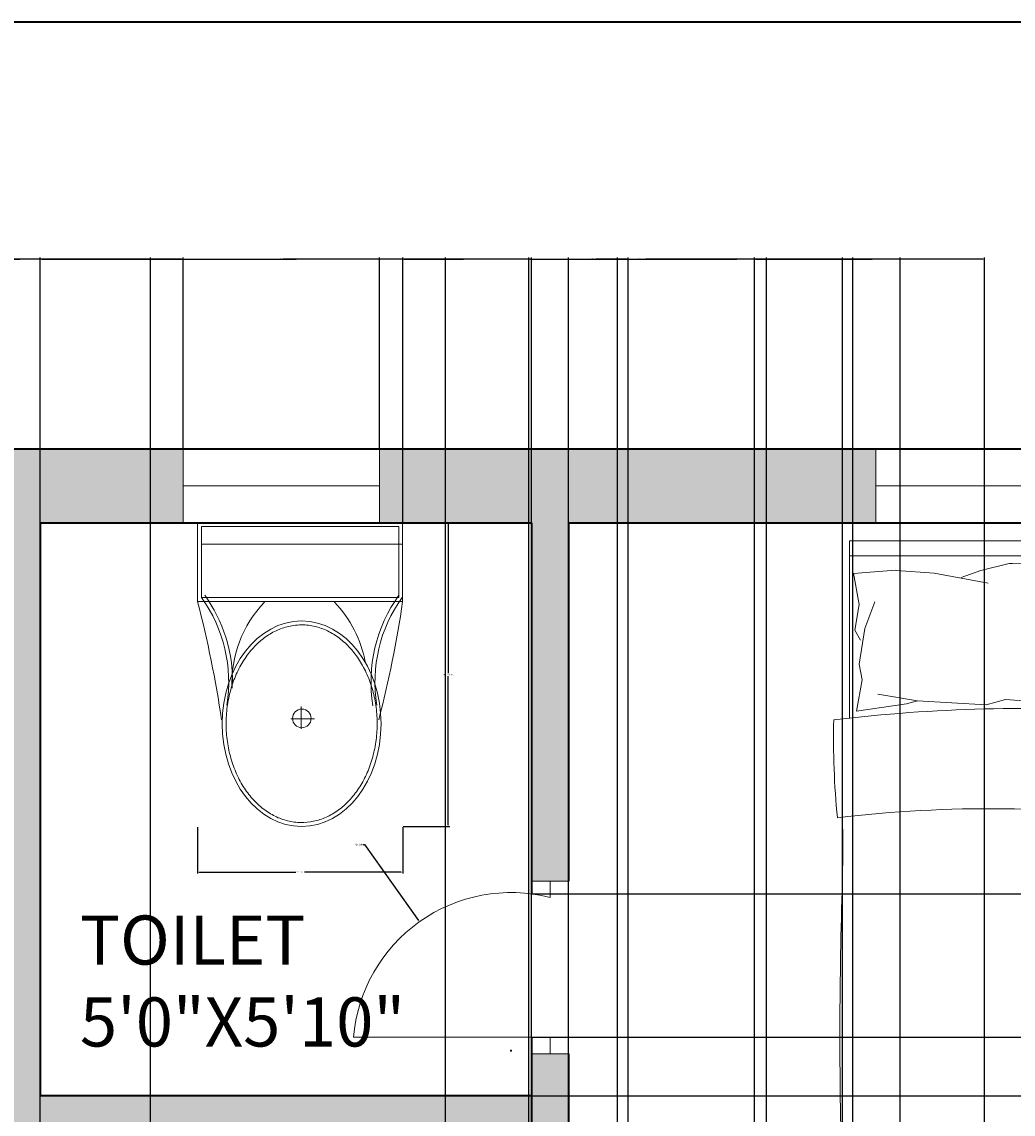
# Model space of a CAD drawing. Units: inches. Extents: x 2606 to 3027, y 1906 to 2463.
# Tile 9 of 10: x 2785 to 2906, y 2329 to 2463. Entities that reach past the tile are written whole.
import ezdxf

# ---------------------------------------------------------------- set-up
doc = ezdxf.new("R2010")
doc.units = ezdxf.units.IN
for name, color, linetype, lineweight in [('A-ANNO-DIMS', 2, 'Continuous', 18), ('A-ANNO-TTLB', 7, 'Continuous', 35), ('A-AREA-IDEN', 7, 'Continuous', 18), ('A-DOOR', 3, 'Continuous', 18), ('A-FLOR-FIXT', 9, 'Continuous', 18), ('A-FURN', 8, 'Continuous', 13), ('A-GLAZ', 4, 'Continuous', 18), ('A-WALL', 7, 'Continuous', 35)]:
    doc.layers.add(name, color=color, linetype=linetype, lineweight=lineweight)
doc.layers.add('A-WALL-PATT', color=251, linetype='Continuous', lineweight=13, true_color=0x636466)
doc.styles.get("Standard").update_dxf_attribs({"font": 'arial.ttf'})
doc.dimstyles.get("Standard").update_dxf_attribs({"dimtxt": 0.18, "dimasz": 0.18, "dimexe": 0.18, "dimexo": 0.0625, "dimgap": 0.09, "dimtad": 0, "dimtih": 1, "dimtoh": 1, "dimdec": 4, "dimzin": 0, "dimdsep": 46, "dimtxsty": 'Standard', "dimcen": 0.09, "dimadec": 0, "dimazin": 0, "dimtfac": 1, "dimtdec": 4, "dimtofl": 0, "dimtmove": 0, "dimatfit": 3, "dimfxl": 1, "dimtolj": 1, "dimtzin": 0, "dimarcsym": 0})

# ---------------------------------------------------------------- blocks, each defined once
blk = doc.blocks.new('A$C31115884')
for p, q in [((257.5, 466.4), (257.5, 523.2)), ((283.1, 497.7), (223.4, 497.7)), ((0, 200), (0, 0)), ((520, 200), (0, 200)), ((520, 0), (520, 200)), ((10, 190), (10, 10)), ((510, 190), (10, 190)), ((510, 10), (510, 190)), ((510, 54.5), (0, 54.5)), ((10, 10), (510, 10)), ((0, 0), (520, 0))]:
    blk.add_line(p, q)
blk.add_circle((255.6, 496.4), 23.6)
for centre, radius, start, end in [((2777.7, -204.6), 2807, 165.4549, 171.7133), ((3237, 905), 2807, 188.2867, 194.5451), ((-294.5, 403.3), 364.7, 324.2091, 9.3499), ((-294.5, 403.3), 374.7, 324.2091, 9.3499), ((805.8, 403.3), 364.7, 170.6501, 215.7909), ((139.5, 406.2), 293.5, 315.8436, 2.6563), ((805.8, 403.3), 374.7, 179.2036, 215.7909), ((383.6, 406.2), 293.5, 190.2774, 224.1564)]:
    blk.add_arc(centre, radius, start, end)
blk.add_ellipse((256.2, 509.9), major_axis=(0, -260.7), ratio=0.772727)
blk.add_open_spline([(256.2, 259.2), (263.1, 259.2), (270, 259.7), (287.8, 262.3), (298.7, 265.1), (319.9, 273.1), (330.2, 278.4), (350.1, 291.1), (359.7, 298.7), (377.7, 315.9), (386.2, 325.5), (401.7, 346.6), (408.8, 358.1), (421.3, 382.5), (426.8, 395.5), (435.9, 422.4), (439.5, 436.4), (444.8, 465.1), (446.5, 479.7), (447.9, 509.2), (447.6, 524), (445, 553.3), (442.7, 567.8), (436.3, 596), (432.1, 609.7), (421.9, 636), (416, 648.6), (402.5, 672.1), (395, 683), (378.6, 703), (369.8, 712.1), (351.1, 728), (341.3, 734.8), (320.9, 746.2), (310.4, 750.7), (288.9, 757.3), (278, 759.4), (256, 761), (245, 760.6), (223.1, 757.2), (212.3, 754.3), (191.1, 746.1), (180.8, 740.7), (160.9, 727.8), (151.4, 720.1), (133.5, 702.7), (125.1, 693), (109.6, 671.7), (102.6, 660.2), (90.2, 635.7), (84.9, 622.7), (76, 595.6), (72.4, 581.6), (67.2, 552.9), (65.6, 538.2), (64.4, 508.8), (64.8, 494), (67.5, 464.7), (69.9, 450.2), (76.6, 422), (80.8, 408.3), (91.1, 382.2), (97.2, 369.7), (110.8, 346.3), (118.4, 335.4), (134.8, 315.6), (143.7, 306.7), (162.4, 290.9), (172.3, 284.2), (192.8, 273), (203.3, 268.6), (224.8, 262.2), (235.8, 260.2), (249.9, 259.3), (253, 259.2), (256.2, 259.2)], degree=3, knots=[0, 0, 0, 0, 0.110105, 0.110105, 0.285049, 0.285049, 0.459994, 0.459994, 0.634938, 0.634938, 0.809882, 0.809882, 0.984827, 0.984827, 1.159771, 1.159771, 1.334715, 1.334715, 1.50966, 1.50966, 1.684604, 1.684604, 1.859549, 1.859549, 2.034493, 2.034493, 2.209437, 2.209437, 2.384382, 2.384382, 2.559326, 2.559326, 2.73427, 2.73427, 2.909215, 2.909215, 3.084159, 3.084159, 3.259103, 3.259103, 3.434048, 3.434048, 3.608992, 3.608992, 3.783936, 3.783936, 3.958881, 3.958881, 4.133825, 4.133825, 4.30877, 4.30877, 4.483714, 4.483714, 4.658658, 4.658658, 4.833603, 4.833603, 5.008547, 5.008547, 5.183491, 5.183491, 5.358436, 5.358436, 5.53338, 5.53338, 5.708324, 5.708324, 5.883269, 5.883269, 6.058213, 6.058213, 6.233158, 6.233158, 6.283185, 6.283185, 6.283185, 6.283185])
blk = doc.blocks.new('BED-DOUBLE')
for p, q in [((4.17, 75.16), (4.17, 96.87)), ((4.17, 96.87), (61.46, 96.87)), ((61.46, 96.87), (61.46, 64.97)), ((4.17, 95.03), (61.46, 95.03)), ((20.24, 93.24), (23.7, 94.11)), ((23.7, 94.11), (24.09, 94.11)), ((24.09, 94.11), (29.42, 93.94)), ((29.42, 93.94), (31.15, 94.63)), ((31.15, 94.63), (31.84, 88.22)), ((33.54, 93.89), (33.25, 87.44)), ((35.31, 93.3), (33.54, 93.89)), ((40.62, 93.81), (35.31, 93.3)), ((41.01, 93.83), (40.62, 93.81)), ((44.52, 93.18), (41.01, 93.83)), ((54.8, 93.82), (50.25, 93.19)), ((60.08, 93.81), (53.6, 93.92)), ((53.6, 93.92), (54.8, 93.82)), ((60.08, 93.81), (59.62, 89.96)), ((4.67, 92.87), (9.81, 93.27)), ((4.67, 92.9), (5.36, 89.08)), ((9.81, 93.27), (9.93, 93.24)), ((9.93, 93.24), (14.52, 92.9)), ((14.52, 92.9), (21.1, 91.68)), ((17.81, 92.38), (20.24, 93.24)), ((50.25, 93.19), (43.75, 91.57)), ((47, 92.47), (44.52, 93.18)), ((6.06, 86.14), (7.27, 89.43)), ((59.12, 86.97), (57.7, 90.18)), ((59.62, 89.96), (60.34, 86.88)), ((5.36, 89.08), (4.84, 85.96)), ((31.84, 88.22), (32.54, 84.4)), ((33.25, 87.44), (32.79, 83.59)), ((60.08, 82.69), (59.12, 86.97)), ((60.34, 86.88), (59.72, 85.62)), ((4.84, 85.96), (5.54, 84.75)), ((5.36, 81.8), (6.06, 86.14)), ((32.54, 84.4), (32.54, 82.84)), ((32.54, 82.84), (31.84, 80.59)), ((32.79, 83.59), (32.89, 82.03)), ((5.71, 79.9), (5.36, 81.8)), ((32.89, 82.03), (33.72, 79.83)), ((59.85, 80.77), (60.08, 82.69)), ((31.84, 80.59), (31.84, 77.38)), ((60.78, 77), (59.85, 80.77)), ((5.02, 76.08), (5.71, 79.9)), ((33.72, 79.83), (33.92, 76.62)), ((7.65, 78.14), (12.48, 77.34)), ((20.89, 76.82), (23.24, 77.49)), ((23.24, 77.49), (29.39, 77)), ((28.9, 77.38), (25.13, 78.68)), ((36.87, 76.8), (40.55, 78.34)), ((39.04, 78.14), (43.87, 77.34)), ((52.28, 76.82), (54.63, 77.49)), ((54.63, 77.49), (60.78, 77)), ((11.13, 76.95), (5.02, 76.08)), ((12.48, 77.34), (11.13, 76.95)), ((12.48, 77.34), (20.89, 76.82)), ((31.84, 77.38), (28.9, 77.38)), ((33.92, 76.62), (36.87, 76.8)), ((43.87, 77.34), (52.28, 76.82)), ((36.28, 76.03), (41.3, 68.25)), ((48.73, 72.52), (38.73, 76.03)), ((55.41, 70.1), (48.73, 72.52)), ((58.94, 67.51), (55.41, 70.1)), ((41.3, 68.25), (43.34, 62.87)), ((63.38, 63.61), (58.94, 67.51)), ((43.34, 62.87), (43.71, 60.45)), ((49.1, 62.31), (53.18, 62.87)), ((53.18, 62.87), (57.82, 63.24)), ((57.82, 63.24), (61.54, 62.87)), ((61.54, 62.87), (63.38, 63.61)), ((63.48, 61.52), (63.38, 63.61, 4.64)), ((46.68, 61.2), (49.1, 62.31)), ((43.71, 60.45), (46.68, 61.2)), ((18.06, 1.87), (47.57, 1.87))]:
    blk.add_line(p, q)
for centre, radius, start, end in [((25.61, -121.38), 197.77, 86.0865, 96.7821), ((102.1, 72.78), 99.87, 178.7218, 185.604), ((21.29, -90.53), 154.68, 81.7845, 96.9006), ((-200.58, 59.5), 203.94, 358.4762, 1.0082), ((37.35, 95.1), 35.55, 280.6617, 289.8806), ((52.44, 54.83), 7.46, 78.6608, 113.7384), ((61.53, 104.85), 43.38, 259.8763, 272.5657), ((218.51, 53.34), 155.25, 176.9791, 183.8365), ((43.92, 60.38), 0.221, 160.2464, 271.1377), ((581.23, 36.19), 578.22, 178.22771, 181.71854), ((-5405.34, 15.56), 5469.02, 0.00217, 0.28689), ((-32.25, 19.53), 35.53, 346.0648, 358.9113), ((91.3, 14.55), 27.65, 177.4714, 206.4681), ((-25.97, 12.62), 28.25, 337.9751, 356.652), ((-20.65, 125.3), 127.63, 283.3832, 287.7053), ((1.3, 1.3), 1.31, 146.1736, 293.4781), ((25.69, -143.9), 145.97, 92.9958, 99.4091), ((49.34, -157.62), 159.5, 84.4998, 90.6351), ((65.23, 2.32), 1.32, 242.6588, 356.02)]:
    blk.add_arc(centre, radius, start, end)
blk = doc.blocks.new('WIN-60IN')
for p, q in [((0, 9), (0, 0)), ((60, 4.5), (60, 9)), ((60, 9), (60, 0)), ((0, 0), (0, 4.5)), ((0, 4.5), (60, 4.5))]:
    blk.add_line(p, q)
blk = doc.blocks.new('*D15')
at = {"layer": 'A-ANNO-DIMS', "color": 0, "lineweight": -2, "transparency": 16777216}
for p, q in [((2831.88, 2401.61), (2837.56, 2401.61)), ((2837.38, 2401.43), (2837.38, 2383.24)), ((2837.38, 2364.68), (2837.38, 2382.87)), ((2831.88, 2364.5), (2837.56, 2364.5))]:
    blk.add_line(p, q, dxfattribs=at)
at = {"layer": 'A-ANNO-DIMS', "color": 0, "transparency": 16777216}
for points in [[(2837.35, 2401.43), (2837.41, 2401.43), (2837.38, 2401.61)], [(2837.35, 2364.68), (2837.41, 2364.68), (2837.38, 2364.5)]]:
    blk.add_solid(points, dxfattribs=at)
at = {"layer": 'Defpoints', "color": 0, "transparency": 16777216}
for p in [(2831.82, 2401.61), (2831.82, 2364.5), (2837.38, 2364.5)]:
    blk.add_point(p, dxfattribs=at)
at = {"layer": 'A-ANNO-DIMS', "color": 0, "transparency": 16777216, "insert": (2837.38, 2383.05), "char_height": 0.18, "attachment_point": 5}
blk.add_mtext('\\A1;WC 37 TYP.', dxfattribs=at)
blk = doc.blocks.new('*D16')
at = {"layer": 'A-ANNO-DIMS', "color": 0, "lineweight": -2, "transparency": 16777216}
for p, q in [((2806.77, 2364.43), (2806.77, 2358.75)), ((2831.82, 2364.43), (2831.82, 2358.75)), ((2806.95, 2358.93), (2818.77, 2358.93)), ((2831.64, 2358.93), (2819.82, 2358.93))]:
    blk.add_line(p, q, dxfattribs=at)
at = {"layer": 'A-ANNO-DIMS', "color": 0, "transparency": 16777216}
for points in [[(2806.95, 2358.96), (2806.95, 2358.9), (2806.77, 2358.93)], [(2831.64, 2358.96), (2831.64, 2358.9), (2831.82, 2358.93)]]:
    blk.add_solid(points, dxfattribs=at)
at = {"layer": 'Defpoints', "color": 0, "transparency": 16777216}
for p in [(2806.77, 2364.5), (2831.82, 2364.5), (2806.77, 2358.93)]:
    blk.add_point(p, dxfattribs=at)
at = {"layer": 'A-ANNO-DIMS', "color": 0, "transparency": 16777216, "insert": (2819.29, 2358.93), "char_height": 0.18, "attachment_point": 5}
blk.add_mtext('\\A1;25 TYP.', dxfattribs=at)
blk = doc.blocks.new('*D28')
at = {"layer": 'A-ANNO-DIMS', "color": 0, "lineweight": -2, "transparency": 16777216}
for p, q in [((2751.97, 2410.67), (2751.97, 2433.99)), ((2752.15, 2433.81), (2778.09, 2433.81)), ((2804.82, 2433.81), (2778.88, 2433.81)), ((2805, 2410.67), (2805, 2433.99))]:
    blk.add_line(p, q, dxfattribs=at)
at = {"layer": 'A-ANNO-DIMS', "color": 0, "transparency": 16777216}
for points in [[(2752.15, 2433.84), (2752.15, 2433.78), (2751.97, 2433.81)], [(2804.82, 2433.84), (2804.82, 2433.78), (2805, 2433.81)]]:
    blk.add_solid(points, dxfattribs=at)
at = {"layer": 'Defpoints', "color": 0, "transparency": 16777216}
for p in [(2805, 2433.81), (2751.97, 2410.61), (2805, 2410.61)]:
    blk.add_point(p, dxfattribs=at)
at = {"layer": 'A-ANNO-DIMS', "color": 0, "transparency": 16777216, "insert": (2778.48, 2433.81), "char_height": 0.18, "attachment_point": 5}
blk.add_mtext('\\A1;53.03', dxfattribs=at)
blk = doc.blocks.new('*D29')
at = {"layer": 'A-ANNO-DIMS', "color": 0, "lineweight": -2, "transparency": 16777216}
for p, q in [((2805, 2410.67), (2805, 2433.99)), ((2805.18, 2433.81), (2816.78, 2433.81)), ((2828.82, 2433.81), (2817.22, 2433.81)), ((2829, 2410.67), (2829, 2433.99))]:
    blk.add_line(p, q, dxfattribs=at)
at = {"layer": 'A-ANNO-DIMS', "color": 0, "transparency": 16777216}
for points in [[(2805.18, 2433.84), (2805.18, 2433.78), (2805, 2433.81)], [(2828.82, 2433.84), (2828.82, 2433.78), (2829, 2433.81)]]:
    blk.add_solid(points, dxfattribs=at)
at = {"layer": 'Defpoints', "color": 0, "transparency": 16777216}
for p in [(2829, 2433.81), (2805, 2410.61), (2829, 2410.61)]:
    blk.add_point(p, dxfattribs=at)
at = {"layer": 'A-ANNO-DIMS', "color": 0, "transparency": 16777216, "insert": (2817, 2433.81), "char_height": 0.18, "attachment_point": 5}
blk.add_mtext('\\A1;24', dxfattribs=at)
blk = doc.blocks.new('*D34')
at = {"layer": 'A-ANNO-DIMS', "color": 0, "lineweight": -2, "transparency": 16777216}
for p, q in [((2787.56, 2118.27), (2787.56, 2433.99)), ((2787.74, 2433.81), (2817.34, 2433.81)), ((2847.38, 2433.81), (2817.78, 2433.81)), ((2847.56, 2118.27), (2847.56, 2433.99))]:
    blk.add_line(p, q, dxfattribs=at)
at = {"layer": 'A-ANNO-DIMS', "color": 0, "transparency": 16777216}
for points in [[(2787.74, 2433.84), (2787.74, 2433.78), (2787.56, 2433.81)], [(2847.38, 2433.84), (2847.38, 2433.78), (2847.56, 2433.81)]]:
    blk.add_solid(points, dxfattribs=at)
at = {"layer": 'Defpoints', "color": 0, "transparency": 16777216}
for p in [(2847.56, 2433.81), (2787.56, 2118.21), (2847.56, 2118.21)]:
    blk.add_point(p, dxfattribs=at)
at = {"layer": 'A-ANNO-DIMS', "color": 0, "transparency": 16777216, "insert": (2817.56, 2433.81), "char_height": 0.18, "attachment_point": 5}
blk.add_mtext('\\A1;60', dxfattribs=at)
blk = doc.blocks.new('*D35')
at = {"layer": 'A-ANNO-DIMS', "color": 0, "lineweight": -2, "transparency": 16777216}
for p, q in [((2801.04, 1993.17), (2801.04, 2433.99)), ((2801.22, 2433.81), (2818.82, 2433.81)), ((2836.86, 2433.81), (2819.26, 2433.81)), ((2837.04, 1993.17), (2837.04, 2433.99))]:
    blk.add_line(p, q, dxfattribs=at)
at = {"layer": 'A-ANNO-DIMS', "color": 0, "transparency": 16777216}
for points in [[(2801.22, 2433.84), (2801.22, 2433.78), (2801.04, 2433.81)], [(2836.86, 2433.84), (2836.86, 2433.78), (2837.04, 2433.81)]]:
    blk.add_solid(points, dxfattribs=at)
at = {"layer": 'Defpoints', "color": 0, "transparency": 16777216}
for p in [(2837.04, 2433.81), (2801.04, 1993.11), (2837.04, 1993.11)]:
    blk.add_point(p, dxfattribs=at)
at = {"layer": 'A-ANNO-DIMS', "color": 0, "transparency": 16777216, "insert": (2819.04, 2433.81), "char_height": 0.18, "attachment_point": 5}
blk.add_mtext('\\A1;36', dxfattribs=at)
blk = doc.blocks.new('*D36')
at = {"layer": 'A-ANNO-DIMS', "color": 0, "lineweight": -2, "transparency": 16777216}
for p, q in [((2787.56, 1993.17), (2787.56, 2433.99)), ((2787.74, 2433.81), (2793.85, 2433.81)), ((2800.86, 2433.81), (2794.76, 2433.81)), ((2801.04, 1993.17), (2801.04, 2433.99))]:
    blk.add_line(p, q, dxfattribs=at)
at = {"layer": 'A-ANNO-DIMS', "color": 0, "transparency": 16777216}
for points in [[(2787.74, 2433.84), (2787.74, 2433.78), (2787.56, 2433.81)], [(2800.86, 2433.84), (2800.86, 2433.78), (2801.04, 2433.81)]]:
    blk.add_solid(points, dxfattribs=at)
at = {"layer": 'Defpoints', "color": 0, "transparency": 16777216}
for p in [(2787.56, 2433.81), (2787.56, 1993.11), (2801.04, 1993.11)]:
    blk.add_point(p, dxfattribs=at)
at = {"layer": 'A-ANNO-DIMS', "color": 0, "transparency": 16777216, "insert": (2794.3, 2433.81), "char_height": 0.18, "attachment_point": 5}
blk.add_mtext('\\A1;13.478', dxfattribs=at)
blk = doc.blocks.new('*D38')
at = {"layer": 'A-ANNO-DIMS', "color": 0, "lineweight": -2, "transparency": 16777216}
for p, q in [((2783.06, 1993.17), (2783.06, 2433.99)), ((2783.24, 2433.81), (2785.05, 2433.81)), ((2787.38, 2433.81), (2785.57, 2433.81)), ((2787.56, 1993.17), (2787.56, 2433.99))]:
    blk.add_line(p, q, dxfattribs=at)
at = {"layer": 'A-ANNO-DIMS', "color": 0, "transparency": 16777216}
for points in [[(2783.24, 2433.84), (2783.24, 2433.78), (2783.06, 2433.81)], [(2787.38, 2433.84), (2787.38, 2433.78), (2787.56, 2433.81)]]:
    blk.add_solid(points, dxfattribs=at)
at = {"layer": 'Defpoints', "color": 0, "transparency": 16777216}
for p in [(2787.56, 2433.81), (2783.06, 1993.11), (2787.56, 1993.11)]:
    blk.add_point(p, dxfattribs=at)
at = {"layer": 'A-ANNO-DIMS', "color": 0, "transparency": 16777216, "insert": (2785.31, 2433.81), "char_height": 0.18, "attachment_point": 5}
blk.add_mtext('\\A1;4.5', dxfattribs=at)
blk = doc.blocks.new('*D44')
at = {"layer": 'A-ANNO-DIMS', "color": 0, "lineweight": -2, "transparency": 16777216}
for p, q in [((2858.06, 2257.67), (2858.06, 2433.99)), ((2858.24, 2433.81), (2871.33, 2433.81)), ((2885.35, 2433.81), (2872.26, 2433.81)), ((2885.53, 2257.67), (2885.53, 2433.99))]:
    blk.add_line(p, q, dxfattribs=at)
at = {"layer": 'A-ANNO-DIMS', "color": 0, "transparency": 16777216}
for points in [[(2858.24, 2433.84), (2858.24, 2433.78), (2858.06, 2433.81)], [(2885.35, 2433.84), (2885.35, 2433.78), (2885.53, 2433.81)]]:
    blk.add_solid(points, dxfattribs=at)
at = {"layer": 'Defpoints', "color": 0, "transparency": 16777216}
for p in [(2885.53, 2433.81), (2858.06, 2257.61), (2885.53, 2257.61)]:
    blk.add_point(p, dxfattribs=at)
at = {"layer": 'A-ANNO-DIMS', "color": 0, "transparency": 16777216, "insert": (2871.79, 2433.81), "char_height": 0.18, "attachment_point": 5}
blk.add_mtext('\\A1;27.475', dxfattribs=at)
blk = doc.blocks.new('*D46')
at = {"layer": 'A-ANNO-DIMS', "color": 0, "lineweight": -2, "transparency": 16777216}
for p, q in [((2859.37, 2154.92), (2859.37, 2433.99)), ((2859.55, 2433.81), (2872.63, 2433.81)), ((2886.63, 2433.81), (2873.56, 2433.81)), ((2886.81, 2157.17), (2886.81, 2433.99))]:
    blk.add_line(p, q, dxfattribs=at)
at = {"layer": 'A-ANNO-DIMS', "color": 0, "transparency": 16777216}
for points in [[(2859.55, 2433.84), (2859.55, 2433.78), (2859.37, 2433.81)], [(2886.63, 2433.84), (2886.63, 2433.78), (2886.81, 2433.81)]]:
    blk.add_solid(points, dxfattribs=at)
at = {"layer": 'Defpoints', "color": 0, "transparency": 16777216}
for p in [(2886.81, 2433.81), (2886.81, 2157.11), (2859.37, 2154.86)]:
    blk.add_point(p, dxfattribs=at)
at = {"layer": 'A-ANNO-DIMS', "color": 0, "transparency": 16777216, "insert": (2873.09, 2433.81), "char_height": 0.18, "attachment_point": 5}
blk.add_mtext('\\A1;27.443', dxfattribs=at)
blk = doc.blocks.new('*D48')
at = {"layer": 'A-ANNO-DIMS', "color": 0, "lineweight": -2, "transparency": 16777216}
for p, q in [((2858.07, 2028.17), (2858.07, 2433.99)), ((2858.25, 2433.81), (2866.77, 2433.81)), ((2876.06, 2433.81), (2867.54, 2433.81)), ((2876.24, 2028.17), (2876.24, 2433.99))]:
    blk.add_line(p, q, dxfattribs=at)
at = {"layer": 'A-ANNO-DIMS', "color": 0, "transparency": 16777216}
for points in [[(2858.25, 2433.84), (2858.25, 2433.78), (2858.07, 2433.81)], [(2876.06, 2433.84), (2876.06, 2433.78), (2876.24, 2433.81)]]:
    blk.add_solid(points, dxfattribs=at)
at = {"layer": 'Defpoints', "color": 0, "transparency": 16777216}
for p in [(2876.24, 2433.81), (2858.07, 2028.11), (2876.24, 2028.11)]:
    blk.add_point(p, dxfattribs=at)
at = {"layer": 'A-ANNO-DIMS', "color": 0, "transparency": 16777216, "insert": (2867.16, 2433.81), "char_height": 0.18, "attachment_point": 5}
blk.add_mtext('\\A1;18.17', dxfattribs=at)
blk = doc.blocks.new('*D49')
at = {"layer": 'A-ANNO-DIMS', "color": 0, "lineweight": -2, "transparency": 16777216}
for p, q in [((2847.63, 2356.26), (3000.44, 2356.26)), ((3000.26, 2356.08), (3000.26, 2347.69)), ((3000.26, 2338.93), (3000.26, 2347.32)), ((2847.63, 2338.75), (3000.44, 2338.75))]:
    blk.add_line(p, q, dxfattribs=at)
at = {"layer": 'A-ANNO-DIMS', "color": 0, "transparency": 16777216}
for points in [[(3000.23, 2356.08), (3000.29, 2356.08), (3000.26, 2356.26)], [(3000.23, 2338.93), (3000.29, 2338.93), (3000.26, 2338.75)]]:
    blk.add_solid(points, dxfattribs=at)
at = {"layer": 'Defpoints', "color": 0, "transparency": 16777216}
for p in [(2847.56, 2356.26), (3000.26, 2356.26), (2847.56, 2338.75)]:
    blk.add_point(p, dxfattribs=at)
at = {"layer": 'A-ANNO-DIMS', "color": 0, "transparency": 16777216, "insert": (3000.26, 2347.51), "char_height": 0.18, "attachment_point": 5}
blk.add_mtext('\\A1;17.516', dxfattribs=at)
blk = doc.blocks.new('*D51')
at = {"layer": 'A-ANNO-DIMS', "color": 0, "lineweight": -2, "transparency": 16777216}
for p, q in [((2852.06, 2257.67), (2852.06, 2433.99)), ((2852.24, 2433.81), (2854.67, 2433.81)), ((2857.88, 2433.81), (2855.45, 2433.81)), ((2858.06, 2257.67), (2858.06, 2433.99))]:
    blk.add_line(p, q, dxfattribs=at)
at = {"layer": 'A-ANNO-DIMS', "color": 0, "transparency": 16777216}
for points in [[(2852.24, 2433.84), (2852.24, 2433.78), (2852.06, 2433.81)], [(2857.88, 2433.84), (2857.88, 2433.78), (2858.06, 2433.81)]]:
    blk.add_solid(points, dxfattribs=at)
at = {"layer": 'Defpoints', "color": 0, "transparency": 16777216}
for p in [(2858.06, 2433.81), (2852.06, 2257.61), (2858.06, 2257.61)]:
    blk.add_point(p, dxfattribs=at)
at = {"layer": 'A-ANNO-DIMS', "color": 0, "transparency": 16777216, "insert": (2855.06, 2433.81), "char_height": 0.18, "attachment_point": 5}
blk.add_mtext('\\A1;5.994', dxfattribs=at)
blk = doc.blocks.new('*D53')
at = {"layer": 'A-ANNO-DIMS', "color": 0, "lineweight": -2, "transparency": 16777216}
for p, q in [((2847.63, 2338.75), (3000.44, 2338.75)), ((3000.26, 2338.57), (3000.26, 2335.36)), ((3000.26, 2331.79), (3000.26, 2335)), ((2847.63, 2331.61), (3000.44, 2331.61))]:
    blk.add_line(p, q, dxfattribs=at)
at = {"layer": 'A-ANNO-DIMS', "color": 0, "transparency": 16777216}
for points in [[(3000.23, 2338.57), (3000.29, 2338.57), (3000.26, 2338.75)], [(3000.23, 2331.79), (3000.29, 2331.79), (3000.26, 2331.61)]]:
    blk.add_solid(points, dxfattribs=at)
at = {"layer": 'Defpoints', "color": 0, "transparency": 16777216}
for p in [(2847.56, 2338.75), (3000.26, 2338.75), (2847.56, 2331.61)]:
    blk.add_point(p, dxfattribs=at)
at = {"layer": 'A-ANNO-DIMS', "color": 0, "transparency": 16777216, "insert": (3000.26, 2335.18), "char_height": 0.18, "attachment_point": 5}
blk.add_mtext('\\A1;7.138', dxfattribs=at)
blk = doc.blocks.new('*D55')
at = {"layer": 'A-ANNO-DIMS', "color": 0, "lineweight": -2, "transparency": 16777216}
for p, q in [((2852.06, 2152.67), (2852.06, 2433.99)), ((2852.24, 2433.81), (2855.32, 2433.81)), ((2859.19, 2433.81), (2856.11, 2433.81)), ((2859.37, 2154.92), (2859.37, 2433.99))]:
    blk.add_line(p, q, dxfattribs=at)
at = {"layer": 'A-ANNO-DIMS', "color": 0, "transparency": 16777216}
for points in [[(2852.24, 2433.84), (2852.24, 2433.78), (2852.06, 2433.81)], [(2859.19, 2433.84), (2859.19, 2433.78), (2859.37, 2433.81)]]:
    blk.add_solid(points, dxfattribs=at)
at = {"layer": 'Defpoints', "color": 0, "transparency": 16777216}
for p in [(2859.37, 2433.81), (2859.37, 2154.86), (2852.06, 2152.61)]:
    blk.add_point(p, dxfattribs=at)
at = {"layer": 'A-ANNO-DIMS', "color": 0, "transparency": 16777216, "insert": (2855.72, 2433.81), "char_height": 0.18, "attachment_point": 5}
blk.add_mtext('\\A1;7.306', dxfattribs=at)
blk = doc.blocks.new('*D57')
at = {"layer": 'A-ANNO-DIMS', "color": 0, "lineweight": -2, "transparency": 16777216}
for p, q in [((2876.24, 2028.17), (2876.24, 2433.99)), ((2876.42, 2433.81), (2889.17, 2433.81)), ((2902.71, 2433.81), (2889.96, 2433.81)), ((2902.89, 2028.17), (2902.89, 2433.99))]:
    blk.add_line(p, q, dxfattribs=at)
at = {"layer": 'A-ANNO-DIMS', "color": 0, "transparency": 16777216}
for points in [[(2876.42, 2433.84), (2876.42, 2433.78), (2876.24, 2433.81)], [(2902.71, 2433.84), (2902.71, 2433.78), (2902.89, 2433.81)]]:
    blk.add_solid(points, dxfattribs=at)
at = {"layer": 'Defpoints', "color": 0, "transparency": 16777216}
for p in [(2902.89, 2433.81), (2876.24, 2028.11), (2902.89, 2028.11)]:
    blk.add_point(p, dxfattribs=at)
at = {"layer": 'A-ANNO-DIMS', "color": 0, "transparency": 16777216, "insert": (2889.57, 2433.81), "char_height": 0.18, "attachment_point": 5}
blk.add_mtext('\\A1;26.65', dxfattribs=at)
blk = doc.blocks.new('*D70')
at = {"layer": 'A-ANNO-DIMS', "color": 0, "lineweight": -2, "transparency": 16777216}
for p, q in [((2847.23, 2221.7), (2847.23, 2433.99)), ((2847.41, 2433.81), (2860.54, 2433.81)), ((2874.6, 2433.81), (2861.47, 2433.81)), ((2874.78, 2221.7), (2874.78, 2433.99))]:
    blk.add_line(p, q, dxfattribs=at)
at = {"layer": 'A-ANNO-DIMS', "color": 0, "transparency": 16777216}
for points in [[(2847.41, 2433.84), (2847.41, 2433.78), (2847.23, 2433.81)], [(2874.6, 2433.84), (2874.6, 2433.78), (2874.78, 2433.81)]]:
    blk.add_solid(points, dxfattribs=at)
at = {"layer": 'Defpoints', "color": 0, "transparency": 16777216}
for p in [(2874.78, 2433.81), (2847.23, 2221.64), (2874.78, 2221.64)]:
    blk.add_point(p, dxfattribs=at)
at = {"layer": 'A-ANNO-DIMS', "color": 0, "transparency": 16777216, "insert": (2861, 2433.81), "char_height": 0.18, "attachment_point": 5}
blk.add_mtext('\\A1;27.555', dxfattribs=at)
blk = doc.blocks.new('*D72')
at = {"layer": 'A-ANNO-DIMS', "color": 0, "lineweight": -2, "transparency": 16777216}
for p, q in [((2874.78, 2221.7), (2874.78, 2433.99)), ((2874.96, 2433.81), (2883.22, 2433.81)), ((2892.38, 2433.81), (2884.13, 2433.81)), ((2892.56, 2215.2), (2892.56, 2433.99))]:
    blk.add_line(p, q, dxfattribs=at)
at = {"layer": 'A-ANNO-DIMS', "color": 0, "transparency": 16777216}
for points in [[(2874.96, 2433.84), (2874.96, 2433.78), (2874.78, 2433.81)], [(2892.38, 2433.84), (2892.38, 2433.78), (2892.56, 2433.81)]]:
    blk.add_solid(points, dxfattribs=at)
at = {"layer": 'Defpoints', "color": 0, "transparency": 16777216}
for p in [(2892.56, 2433.81), (2874.78, 2221.64), (2892.56, 2215.13)]:
    blk.add_point(p, dxfattribs=at)
at = {"layer": 'A-ANNO-DIMS', "color": 0, "transparency": 16777216, "insert": (2883.67, 2433.81), "char_height": 0.18, "attachment_point": 5}
blk.add_mtext('\\A1;17.783', dxfattribs=at)
blk = doc.blocks.new('*D82')
at = {"layer": 'A-ANNO-DIMS', "color": 0, "lineweight": -2, "transparency": 16777216}
for p, q in [((2831.82, 2401.67), (2831.82, 2433.99)), ((2832, 2433.81), (2839.24, 2433.81)), ((2847.38, 2433.81), (2840.15, 2433.81)), ((2847.56, 2401.67), (2847.56, 2433.99))]:
    blk.add_line(p, q, dxfattribs=at)
at = {"layer": 'A-ANNO-DIMS', "color": 0, "transparency": 16777216}
for points in [[(2832, 2433.84), (2832, 2433.78), (2831.82, 2433.81)], [(2847.38, 2433.84), (2847.38, 2433.78), (2847.56, 2433.81)]]:
    blk.add_solid(points, dxfattribs=at)
at = {"layer": 'Defpoints', "color": 0, "transparency": 16777216}
for p in [(2847.56, 2433.81), (2831.82, 2401.61), (2847.56, 2401.61)]:
    blk.add_point(p, dxfattribs=at)
at = {"layer": 'A-ANNO-DIMS', "color": 0, "transparency": 16777216, "insert": (2839.69, 2433.81), "char_height": 0.18, "attachment_point": 5}
blk.add_mtext('\\A1;15.746', dxfattribs=at)
blk = doc.blocks.new('*D90')
at = {"layer": 'A-ANNO-DIMS', "color": 0, "lineweight": -2, "transparency": 16777216}
for p, q in [((2826.96, 2362.29), (2827.14, 2362.29)), ((2827.14, 2362.29), (2833.75, 2353)), ((2844.96, 2337.12), (2845.14, 2337.12)), ((2845.05, 2337.03), (2845.05, 2337.21))]:
    blk.add_line(p, q, dxfattribs=at)
at = {"layer": 'A-ANNO-DIMS', "color": 0, "transparency": 16777216}
blk.add_solid([(2833.77, 2353.01), (2833.73, 2352.98), (2833.85, 2352.85)], dxfattribs=at)
at = {"layer": 'Defpoints', "color": 0, "transparency": 16777216}
for p in [(2833.85, 2352.85), (2845.05, 2337.12)]:
    blk.add_point(p, dxfattribs=at)
at = {"layer": 'A-ANNO-DIMS', "color": 0, "transparency": 16777216, "insert": (2826.41, 2362.29), "char_height": 0.18, "attachment_point": 5}
blk.add_mtext('\\A1;R19.305', dxfattribs=at)

msp = doc.modelspace()

# ---------------------------------------------------------------- hatches: boundary and pattern name
at = {"layer": 'A-WALL-PATT'}
h = msp.add_hatch(color=256, dxfattribs=at)
h.dxf.hatch_style = 1
h.paths.add_polyline_path([(2667.063, 2401.6097), (2691.9697, 2401.6097), (2691.9697, 2406.1097), (2691.9697, 2410.6097), (2658.063, 2410.6097), (2658.063, 2238.7051), (2667.063, 2238.7051)])
h.paths.add_polyline_path([(2804.9965, 2406.1097), (2804.9965, 2410.6097), (2751.9697, 2410.6097), (2751.9697, 2401.6097), (2783.063, 2401.6097), (2783.063, 2257.6097), (2778.6739, 2257.6097), (2778.6739, 2253.1097), (2792.3386, 2253.1097), (2792.3386, 2255.3597), (2792.3386, 2257.6097), (2787.563, 2257.6097), (2787.563, 2327.1097), (2847.563, 2327.1097), (2847.563, 2331.6097), (2787.563, 2331.6097), (2787.563, 2401.6097), (2804.9965, 2401.6097)])
h.paths.add_polyline_path([(2889.6183, 2406.1097), (2889.6183, 2410.6097), (2828.9965, 2410.6097), (2828.9965, 2401.6097), (2831.8174, 2401.6097), (2847.563, 2401.6097), (2847.563, 2357.8311), (2849.813, 2357.8311), (2852.063, 2357.8311), (2852.063, 2401.6097), (2889.6183, 2401.6097)])
h.paths.add_polyline_path([(2977.063, 2410.6097), (2949.6183, 2410.6097), (2949.6183, 2401.6097), (2968.063, 2401.6097), (2968.063, 2157.1097), (2897.063, 2157.1097), (2897.063, 2174.1966), (2892.563, 2174.1966), (2892.563, 2157.1097), (2886.8122, 2157.1097), (2886.8122, 2152.6097), (2968.063, 2152.6097), (2968.063, 2032.6097), (2950.8911, 2032.6097), (2950.8911, 2028.1097), (2968.063, 2028.1097), (2968.063, 1993.1097), (2852.063, 1993.1097), (2852.063, 2028.1097), (2856.0743, 2028.1097), (2856.0743, 2030.3597), (2856.0743, 2032.6097), (2852.063, 2032.6097), (2852.063, 2152.6097), (2857.369, 2152.6097), (2857.369, 2154.8597), (2857.369, 2157.1097), (2847.563, 2157.1097), (2847.563, 2152.6097), (2847.563, 1993.1097), (2837.0415, 1993.1097), (2837.0415, 1988.6097), (2977.063, 1988.6097)])
h.paths.add_polyline_path([(2968.063, 2257.6097), (2886.9679, 2257.6097), (2886.9679, 2253.1097), (2892.563, 2253.1097), (2892.563, 2215.1332), (2897.063, 2215.1332), (2897.063, 2253.1097), (2968.063, 2253.1097)], flags=17)
h.paths.add_polyline_path([(2856.057, 2255.3597), (2856.057, 2257.6097), (2852.063, 2257.6097), (2852.063, 2336.7476), (2849.813, 2336.7476), (2847.563, 2336.7476), (2847.563, 2331.6097), (2847.563, 2327.1097), (2847.563, 2257.6097), (2813.482, 2257.6097), (2813.482, 2253.1097), (2856.057, 2253.1097)])
h.paths.add_polyline_path([(2748.8874, 2255.3597), (2748.8874, 2257.6097), (2667.063, 2257.6097), (2667.063, 2253.1097), (2748.8874, 2253.1097)])
h.paths.add_polyline_path([(2667.063, 2152.6097), (2744.8238, 2152.6097), (2744.8238, 2154.8597), (2744.8238, 2157.1097), (2667.063, 2157.1097), (2667.063, 2178.7051), (2658.063, 2178.7051), (2658.063, 1988.6097), (2801.0415, 1988.6097), (2801.0415, 1990.8597), (2801.0415, 1993.1097), (2787.563, 1993.1097), (2787.563, 2157.1097), (2777.1295, 2157.1097), (2777.1295, 2152.6097), (2783.063, 2152.6097), (2783.063, 2032.6097), (2778.4484, 2032.6097), (2778.4484, 2028.1097), (2783.063, 2028.1097), (2783.063, 1993.1097), (2667.063, 1993.1097), (2667.063, 2028.1097), (2680.1652, 2028.1097), (2680.1652, 2030.3597), (2680.1652, 2032.6097), (2667.063, 2032.6097)])
h.paths.add_polyline_path([(2755.4074, 2032.6097), (2728.1652, 2032.6097), (2728.1652, 2028.1097), (2755.4074, 2028.1097), (2755.4074, 2030.3597)], flags=17)
h.paths.add_polyline_path([(2902.8911, 2030.3597), (2902.8911, 2032.6097), (2877.6885, 2032.6097), (2877.6885, 2028.1097), (2902.8911, 2028.1097)], flags=17)
h.paths.add_polyline_path([(2810.2211, 2267.221), (2851.2716, 2267.221), (2851.2716, 2289.6098), (2810.2211, 2289.6098)], flags=9)
h = msp.add_hatch(color=256, dxfattribs=at)
h.dxf.hatch_style = 1
h.paths.add_polyline_path([(2852.063, 2336.7476), (2849.813, 2336.7476), (2847.563, 2336.7476), (2847.563, 2331.6097), (2847.563, 2257.6097), (2813.482, 2257.6097), (2813.482, 2253.1097), (2856.057, 2253.1097), (2856.057, 2255.3597), (2856.057, 2257.6097), (2852.063, 2257.6097)])

# ---------------------------------------------------------------- linework, layer by layer
at = {"layer": 'A-ANNO-TTLB'}
msp.add_lwpolyline([(2605.9227, 2462.7868), (3027.4339, 2462.7868), (3027.4339, 1905.5336), (2605.9227, 1905.5336)], close=True, dxfattribs=at)
at = {"layer": 'A-DOOR'}
for p, q in [((2852.063, 2357.8311), (2847.563, 2357.8311)), ((2847.563, 2357.8311), (2849.813, 2357.8311)), ((2849.813, 2357.8311), (2849.813, 2355.8311)), ((2849.813, 2338.7476), (2825.813, 2338.7476)), ((2849.813, 2336.7476), (2849.813, 2338.7476)), ((2847.563, 2336.7476), (2852.063, 2336.7476)), ((2852.063, 2336.7476), (2849.813, 2336.7476))]:
    msp.add_line(p, q, dxfattribs=at)
msp.add_arc((2845.0492, 2337.1235), 19.3047, 75.713651, 175.173832, dxfattribs=at)
at = {"layer": 'A-GLAZ'}
for p, q in [((2804.9965, 2410.6097), (2804.9965, 2401.6097)), ((2828.9965, 2406.1097), (2828.9965, 2410.6097)), ((2828.9965, 2410.6097), (2828.9965, 2401.6097)), ((2804.9965, 2401.6097), (2804.9965, 2406.1097)), ((2804.9965, 2406.1097), (2828.9965, 2406.1097))]:
    msp.add_line(p, q, dxfattribs=at)
at = {"layer": 'A-WALL'}
for p, q in [((2658.063, 2410.6097), (2977.063, 2410.6097)), ((2787.563, 2401.6097), (2787.563, 2331.6097)), ((2787.563, 2401.6097), (2847.563, 2401.6097)), ((2847.563, 2401.6097), (2847.563, 2356.2638)), ((2847.563, 2401.6097), (2847.563, 2356.2638)), ((2852.063, 2401.6097), (2852.063, 2357.8311)), ((2852.063, 2401.6097), (2968.063, 2401.6097)), ((2847.563, 2338.7476), (2847.563, 2331.6097)), ((2847.563, 2338.7476), (2847.563, 2257.6097)), ((2852.063, 2336.7476), (2852.063, 2257.6097)), ((2847.563, 2331.6097), (2787.563, 2331.6097))]:
    msp.add_line(p, q, dxfattribs=at)

# ---------------------------------------------------------------- block references
at = {"layer": 'A-FLOR-FIXT', "xscale": 0.048164045903398, "yscale": 0.048164045903398, "zscale": 0.048164045903398, "rotation": 180}
msp.add_blockref('A$C31115884', (2831.8174, 2401.6097), dxfattribs=at)
at = {"layer": 'A-FURN'}
msp.add_blockref('BED-DOUBLE', (2882.206, 2302.524), dxfattribs=at)
at = {"layer": 'A-GLAZ'}
msp.add_blockref('WIN-60IN', (2889.6187, 2401.61), dxfattribs=at)

# ---------------------------------------------------------------- texts
at = {"layer": 'A-AREA-IDEN', "insert": (2792.4062, 2353.6252), "char_height": 6, "attachment_point": 1}
msp.add_mtext_dynamic_manual_height_columns('TOILET\\P5\'0"X5\'10"', width=52.081144, gutter_width=12.5, heights=[0], dxfattribs=at)

# ---------------------------------------------------------------- dimensions: what is measured, and where the dimension line sits
at = {"layer": 'A-ANNO-DIMS'}
for base, p1, p2, override, picture, middle in [((2804.9965, 2433.8097), (2751.9697, 2410.6097), (2804.9965, 2410.6097), {"dimdec": 2, "dimlfac": 1, "dimrnd": 0, "dimzin": 0, "dimdsep": 46, "dimlunit": 2}, '*D28', (2778.4831, 2433.8097)), ((2787.563, 2433.8097), (2783.063, 1993.1097), (2787.563, 1993.1097), {"dimdec": 1, "dimlfac": 1, "dimrnd": 0, "dimzin": 0, "dimdsep": 46, "dimlunit": 2}, '*D38', (2785.313, 2433.8097)), ((2847.563, 2433.8097), (2787.563, 2118.2123), (2847.563, 2118.2123), {"dimdec": 0, "dimlfac": 1, "dimrnd": 0, "dimzin": 0, "dimdsep": 46, "dimlunit": 2}, '*D34', (2817.563, 2433.8097)), ((2787.56299, 2433.8097), (2801.04146, 1993.1097), (2787.56299, 1993.1097), {"dimdec": 3, "dimlfac": 1, "dimrnd": 0, "dimzin": 0, "dimdsep": 46, "dimlunit": 2}, '*D36', (2794.30223, 2433.8097)), ((2837.0415, 2433.8097), (2801.0415, 1993.1097), (2837.0415, 1993.1097), {"dimdec": 0, "dimlfac": 1, "dimrnd": 0, "dimzin": 0, "dimdsep": 46, "dimlunit": 2}, '*D35', (2819.0415, 2433.8097)), ((2828.9965, 2433.8097), (2804.9965, 2410.6097), (2828.9965, 2410.6097), {"dimdec": 0, "dimlfac": 1, "dimrnd": 0, "dimzin": 0, "dimdsep": 46, "dimlunit": 2}, '*D29', (2816.9965, 2433.8097)), ((2847.563, 2433.8097), (2831.8174, 2401.6097), (2847.563, 2401.6097), {"dimdec": 3, "dimlfac": 1, "dimrnd": 0, "dimzin": 0, "dimdsep": 46, "dimlunit": 2}, '*D82', (2839.6902, 2433.8097)), ((2874.7801, 2433.8097), (2847.2251, 2221.6399), (2874.7801, 2221.6399), {"dimdec": 3, "dimlfac": 1, "dimrnd": 0, "dimzin": 0, "dimdsep": 46, "dimlunit": 2}, '*D70', (2861.0026, 2433.8097)), ((2858.057, 2433.8097), (2852.063, 2257.6097), (2858.057, 2257.6097), {"dimdec": 3, "dimlfac": 1, "dimrnd": 0, "dimzin": 0, "dimdsep": 46, "dimlunit": 2}, '*D51', (2855.06, 2433.8097)), ((2859.369, 2433.8097), (2852.063, 2152.6097), (2859.369, 2154.8597), {"dimdec": 3, "dimlfac": 1, "dimrnd": 0, "dimzin": 0, "dimdsep": 46, "dimlunit": 2}, '*D55', (2855.716, 2433.8097)), ((2885.5319, 2433.8097), (2858.057, 2257.6097), (2885.5319, 2257.6097), {"dimdec": 3, "dimlfac": 1, "dimrnd": 0, "dimzin": 0, "dimdsep": 46, "dimlunit": 2}, '*D44', (2871.7945, 2433.8097)), ((2876.2433, 2433.8097), (2858.0743, 2028.1097), (2876.2433, 2028.1097), {"dimdec": 2, "dimlfac": 1, "dimrnd": 0, "dimzin": 0, "dimdsep": 46, "dimlunit": 2}, '*D48', (2867.1588, 2433.8097)), ((2886.8122, 2433.8097), (2859.369, 2154.8597), (2886.8122, 2157.1097), {"dimdec": 3, "dimlfac": 1, "dimrnd": 0, "dimzin": 0, "dimdsep": 46, "dimlunit": 2}, '*D46', (2873.0906, 2433.8097)), ((2892.563, 2433.8097), (2874.7801, 2221.6399), (2892.563, 2215.1332), {"dimdec": 3, "dimlfac": 1, "dimrnd": 0, "dimzin": 0, "dimdsep": 46, "dimlunit": 2}, '*D72', (2883.6716, 2433.8097)), ((2902.8911, 2433.8097), (2876.2433, 2028.1097), (2902.8911, 2028.1097), {"dimdec": 2, "dimlfac": 1, "dimrnd": 0, "dimzin": 0, "dimdsep": 46, "dimlunit": 2}, '*D57', (2889.5672, 2433.8097))]:
    dim = msp.add_linear_dim(base=base, p1=p1, p2=p2, dimstyle='Standard', override=override, dxfattribs=at)
    dim.commit()
    dim.dimension.update_dxf_attribs({"geometry": picture, "text_midpoint": middle})
for base, p1, p2, angle, text, picture, middle in [((2837.3845, 2364.4959), (2831.8174, 2401.6097), (2831.8174, 2364.4959), 270, 'WC <> TYP.', '*D15', (2837.3845, 2383.0528)), ((2806.7721, 2358.9289), (2831.8174, 2364.4959), (2806.7721, 2364.4959), 180, '<> TYP.', '*D16', (2819.2948, 2358.9289))]:
    dim = msp.add_linear_dim(base=base, p1=p1, p2=p2, angle=angle, text=text, dimstyle='Standard', override={"dimdec": 0, "dimlfac": 1, "dimrnd": 0, "dimzin": 0, "dimdsep": 46, "dimlunit": 2}, dxfattribs=at)
    dim.commit()
    dim.dimension.update_dxf_attribs({"geometry": picture, "text_midpoint": middle})
dim = msp.add_radius_dim(center=(2845.0492, 2337.1235), mpoint=(2833.8543, 2352.8506), dimstyle='Standard', override={"dimdec": 3, "dimlfac": 1, "dimrnd": 0, "dimzin": 0, "dimdsep": 46, "dimlunit": 2}, dxfattribs=at)
dim.commit()
dim.dimension.update_dxf_attribs({"geometry": '*D90', "text_midpoint": (2826.4069, 2362.2869), "dimtype": 164})
for base, p1, p2, picture, middle in [((3000.263, 2356.2638), (2847.563, 2338.7476), (2847.563, 2356.2638), '*D49', (3000.263, 2347.5057)), ((3000.263, 2338.7476), (2847.563, 2331.6097), (2847.563, 2338.7476), '*D53', (3000.263, 2335.1787))]:
    dim = msp.add_linear_dim(base=base, p1=p1, p2=p2, angle=90, dimstyle='Standard', override={"dimdec": 3, "dimlfac": 1, "dimrnd": 0, "dimzin": 0, "dimdsep": 46, "dimlunit": 2}, dxfattribs=at)
    dim.commit()
    dim.dimension.update_dxf_attribs({"geometry": picture, "text_midpoint": middle})

doc.saveas('drawing.dxf')
